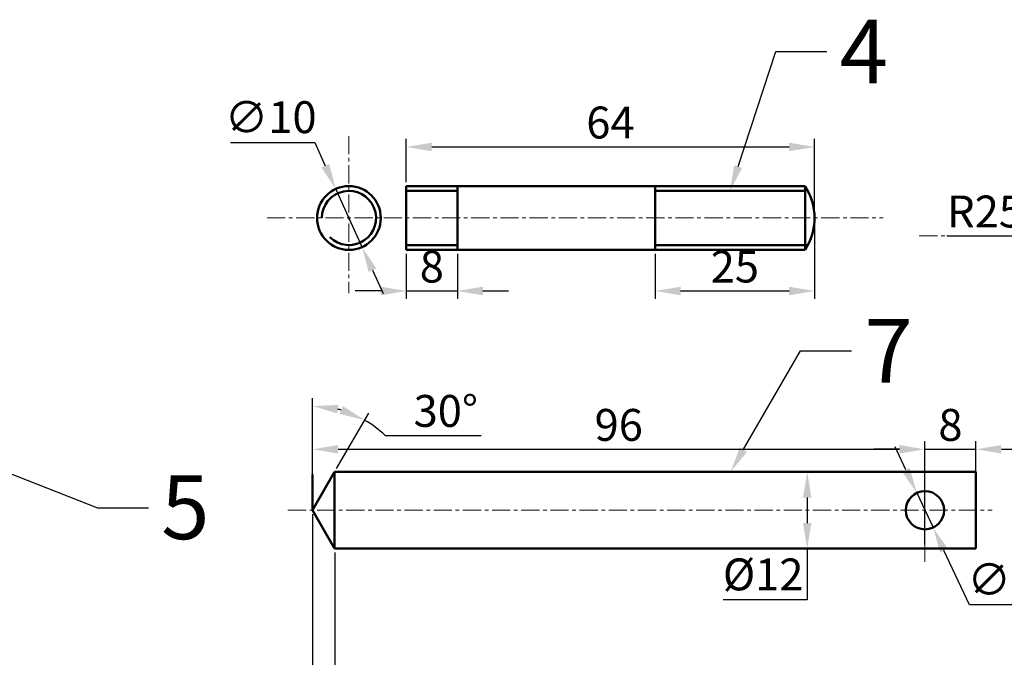
# Model space of a CAD drawing. Units: millimetres. Extents: x 24 to 508, y -182 to 223.
# Tile 4 of 6: x 207 to 361, y -25 to 75. Entities that reach past the tile are written whole.
import ezdxf
from ezdxf import colors
from ezdxf.entities.mleader import LeaderData, LeaderLine
from ezdxf.math import Vec2, Vec3

# ---------------------------------------------------------------- set-up
doc = ezdxf.new("R2010")
doc.units = ezdxf.units.MM
doc.header["$LTSCALE"] = 0.3
doc.linetypes.add('CENTER', pattern=[50.8, 31.75, -6.35, 6.35, -6.35])
for name, color, linetype, lineweight in [('M-CNTR', 1, 'CENTER', 18), ('M-DIMS', 2, 'Continuous', 25), ('M-OUTL', 7, 'Continuous', 50)]:
    doc.layers.add(name, color=color, linetype=linetype, lineweight=lineweight)
doc.styles.get("Standard").update_dxf_attribs({"font": 'arial.ttf'})
doc.dimstyles.new('ISO-25', dxfattribs={"dimtxt": 5, "dimasz": 4, "dimexe": 1.25, "dimexo": 0.625, "dimtad": 1, "dimtoh": 1, "dimdec": 0, "dimtxsty": 'Standard', "dimcen": 2.5, "dimadec": 0, "dimazin": 0, "dimtfac": 1, "dimtdec": 0, "dimtmove": 0, "dimatfit": 3, "dimfxl": 1, "dimarcsym": 0})

# ---------------------------------------------------------------- blocks, each defined once
blk = doc.blocks.new('*D30')
at = {"layer": 'Defpoints', "color": 0, "ltscale": 0.3, "transparency": 16777216}
for p in [(267.18, 38.45), (275.18, 38.45), (275.18, 32)]:
    blk.add_point(p, dxfattribs=at)
at = {"layer": 'M-DIMS', "color": 0, "lineweight": -2, "ltscale": 0.3, "transparency": 16777216}
for p, q in [((267.18, 37.82), (267.18, 30.75)), ((275.18, 37.82), (275.18, 30.75)), ((263.18, 32), (259.18, 32)), ((267.18, 32), (275.18, 32)), ((279.18, 32), (283.18, 32))]:
    blk.add_line(p, q, dxfattribs=at)
at = {"layer": 'M-DIMS', "color": 0, "ltscale": 0.3, "transparency": 16777216}
for points in [[(263.18, 32.67), (263.18, 31.33), (267.18, 32)], [(279.18, 32.67), (279.18, 31.33), (275.18, 32)]]:
    blk.add_solid(points, dxfattribs=at)
at = {"layer": 'M-DIMS', "color": 0, "ltscale": 0.3, "transparency": 16777216, "insert": (271.18, 35.18), "char_height": 5, "attachment_point": 5}
blk.add_mtext('8', dxfattribs=at)
blk = doc.blocks.new('*D31')
at = {"layer": 'Defpoints', "color": 0, "ltscale": 0.3, "transparency": 16777216}
for p in [(331.18, 43.45), (306.18, 38.45), (331.18, 32)]:
    blk.add_point(p, dxfattribs=at)
at = {"layer": 'M-DIMS', "color": 0, "lineweight": -2, "ltscale": 0.3, "transparency": 16777216}
for p, q in [((331.18, 42.82), (331.18, 30.75)), ((306.18, 37.82), (306.18, 30.75)), ((310.18, 32), (327.18, 32))]:
    blk.add_line(p, q, dxfattribs=at)
at = {"layer": 'M-DIMS', "color": 0, "ltscale": 0.3, "transparency": 16777216}
for points in [[(310.18, 32.67), (310.18, 31.33), (306.18, 32)], [(327.18, 32.67), (327.18, 31.33), (331.18, 32)]]:
    blk.add_solid(points, dxfattribs=at)
at = {"layer": 'M-DIMS', "color": 0, "ltscale": 0.3, "transparency": 16777216, "insert": (318.68, 35.18), "char_height": 5, "attachment_point": 5}
blk.add_mtext('25', dxfattribs=at)
blk = doc.blocks.new('*D32')
at = {"layer": 'Defpoints', "color": 0, "ltscale": 0.3, "transparency": 16777216}
for p in [(331.18, 54.59), (267.18, 48.45), (331.18, 43.45)]:
    blk.add_point(p, dxfattribs=at)
at = {"layer": 'M-DIMS', "color": 0, "lineweight": -2, "ltscale": 0.3, "transparency": 16777216}
for p, q in [((267.18, 49.07), (267.18, 55.84)), ((331.18, 44.07), (331.18, 55.84)), ((271.18, 54.59), (327.18, 54.59))]:
    blk.add_line(p, q, dxfattribs=at)
at = {"layer": 'M-DIMS', "color": 0, "ltscale": 0.3, "transparency": 16777216}
for points in [[(271.18, 55.26), (271.18, 53.92), (267.18, 54.59)], [(327.18, 55.26), (327.18, 53.92), (331.18, 54.59)]]:
    blk.add_solid(points, dxfattribs=at)
at = {"layer": 'M-DIMS', "color": 0, "ltscale": 0.3, "transparency": 16777216, "insert": (299.18, 57.77), "char_height": 5, "attachment_point": 5}
blk.add_mtext('64', dxfattribs=at)
blk = doc.blocks.new('*D33')
at = {"layer": 'Defpoints', "color": 0, "ltscale": 0.3, "transparency": 16777216}
for p in [(256.12, 48), (260.24, 38.89)]:
    blk.add_point(p, dxfattribs=at)
at = {"layer": 'M-DIMS', "color": 0, "lineweight": -2, "ltscale": 0.3, "transparency": 16777216}
for p, q in [((239.62, 55.3), (252.83, 55.3)), ((252.83, 55.3), (254.48, 51.65)), ((260.24, 38.89), (256.12, 48)), ((261.88, 35.24), (263.53, 31.6))]:
    blk.add_line(p, q, dxfattribs=at)
at = {"layer": 'M-DIMS', "color": 0, "ltscale": 0.3, "transparency": 16777216}
for points in [[(255.09, 51.92), (253.87, 51.38), (256.12, 48)], [(262.49, 35.52), (261.28, 34.97), (260.24, 38.89)]]:
    blk.add_solid(points, dxfattribs=at)
at = {"layer": 'M-DIMS', "color": 0, "ltscale": 0.3, "transparency": 16777216, "insert": (245.92, 58.61), "char_height": 5, "attachment_point": 5}
blk.add_mtext('∅10', dxfattribs=at)
blk = doc.blocks.new('*D34')
at = {"layer": 'Defpoints', "color": 0, "ltscale": 0.3, "transparency": 16777216}
for p in [(255.32, 13.71), (252.48, 3.24), (255.95, 3.61), (252.48, -2.39), (252.48, -2.39)]:
    blk.add_point(p, dxfattribs=at)
at = {"layer": 'M-DIMS', "color": 0, "lineweight": -2, "ltscale": 0.3, "transparency": 16777216}
for p, q in [((252.48, 3.87), (252.48, 15.2)), ((256.26, 4.16), (261.28, 12.85)), ((263.85, 9.36), (278.9, 9.36))]:
    blk.add_line(p, q, dxfattribs=at)
for start, end in [(74.0616, 75.9384), (45.9384, 60)]:
    blk.add_arc((252.48, -2.39), 16.34, start, end, dxfattribs=at)
at = {"layer": 'M-DIMS', "color": 0, "ltscale": 0.3, "transparency": 16777216}
for points in [[(256.37, 12.8), (256.53, 14.13), (252.48, 13.95)], [(257.23, 13.94), (256.71, 12.71), (260.65, 11.77)]]:
    blk.add_solid(points, dxfattribs=at)
at = {"layer": 'M-DIMS', "color": 0, "ltscale": 0.3, "transparency": 16777216, "insert": (273.37, 12.54), "char_height": 5, "attachment_point": 5}
blk.add_mtext('30°', dxfattribs=at)
blk = doc.blocks.new('*D35')
at = {"layer": 'Defpoints', "color": 0, "ltscale": 0.3, "transparency": 16777216}
for p in [(348.48, 7.17), (252.48, -2.39), (348.48, -2.39)]:
    blk.add_point(p, dxfattribs=at)
at = {"layer": 'M-DIMS', "color": 0, "lineweight": -2, "ltscale": 0.3, "transparency": 16777216}
for p, q in [((252.48, -1.76), (252.48, 8.42)), ((348.48, -1.77), (348.48, 8.42)), ((256.48, 7.17), (344.48, 7.17))]:
    blk.add_line(p, q, dxfattribs=at)
at = {"layer": 'M-DIMS', "color": 0, "ltscale": 0.3, "transparency": 16777216}
for points in [[(256.48, 7.84), (256.48, 6.51), (252.48, 7.17)], [(344.48, 7.84), (344.48, 6.51), (348.48, 7.17)]]:
    blk.add_solid(points, dxfattribs=at)
at = {"layer": 'M-DIMS', "color": 0, "ltscale": 0.3, "transparency": 16777216, "insert": (300.48, 10.35), "char_height": 5, "attachment_point": 5}
blk.add_mtext('96', dxfattribs=at)
blk = doc.blocks.new('*D36')
at = {"layer": 'Defpoints', "color": 0, "ltscale": 0.3, "transparency": 16777216}
for p in [(356.48, 7.17), (348.48, -8.39), (356.48, -8.39)]:
    blk.add_point(p, dxfattribs=at)
at = {"layer": 'M-DIMS', "color": 0, "lineweight": -2, "ltscale": 0.3, "transparency": 16777216}
for p, q in [((348.48, -7.76), (348.48, 8.42)), ((356.48, -7.76), (356.48, 8.42)), ((344.48, 7.17), (340.48, 7.17)), ((348.48, 7.17), (356.48, 7.17)), ((360.48, 7.17), (364.48, 7.17))]:
    blk.add_line(p, q, dxfattribs=at)
at = {"layer": 'M-DIMS', "color": 0, "ltscale": 0.3, "transparency": 16777216}
for points in [[(344.48, 7.84), (344.48, 6.51), (348.48, 7.17)], [(360.48, 7.84), (360.48, 6.51), (356.48, 7.17)]]:
    blk.add_solid(points, dxfattribs=at)
at = {"layer": 'M-DIMS', "color": 0, "ltscale": 0.3, "transparency": 16777216, "insert": (352.48, 10.35), "char_height": 5, "attachment_point": 5}
blk.add_mtext('8', dxfattribs=at)
blk = doc.blocks.new('*D37')
at = {"layer": 'Defpoints', "color": 0, "ltscale": 0.3, "transparency": 16777216}
for p in [(330.03, 3.61), (332.02, 3.61), (332.02, -8.39)]:
    blk.add_point(p, dxfattribs=at)
at = {"layer": 'M-DIMS', "color": 0, "lineweight": -2, "ltscale": 0.3, "transparency": 16777216}
for p, q in [((331.39, 3.61), (328.78, 3.61)), ((330.03, -0.39), (330.03, -4.39)), ((331.39, -8.39), (328.78, -8.39)), ((330.03, -8.39), (330.03, -16.42)), ((330.03, -16.42), (316.85, -16.42))]:
    blk.add_line(p, q, dxfattribs=at)
at = {"layer": 'M-DIMS', "color": 0, "ltscale": 0.3, "transparency": 16777216}
for points in [[(329.36, -0.39), (330.69, -0.39), (330.03, 3.61)], [(329.36, -4.39), (330.69, -4.39), (330.03, -8.39)]]:
    blk.add_solid(points, dxfattribs=at)
at = {"layer": 'M-DIMS', "color": 0, "ltscale": 0.3, "transparency": 16777216, "insert": (323.12, -13.1), "char_height": 5, "attachment_point": 5}
blk.add_mtext('%%C12', dxfattribs=at)
blk = doc.blocks.new('*D38')
at = {"layer": 'Defpoints', "color": 0, "ltscale": 0.3, "transparency": 16777216}
for p in [(347.2, 0.33), (349.76, -5.1)]:
    blk.add_point(p, dxfattribs=at)
at = {"layer": 'M-DIMS', "color": 0, "lineweight": -2, "ltscale": 0.3, "transparency": 16777216}
for p, q in [((345.5, 3.95), (343.8, 7.57)), ((347.2, 0.33), (349.76, -5.1)), ((355.46, -17.21), (351.47, -8.72)), ((364.8, -17.21), (355.46, -17.21))]:
    blk.add_line(p, q, dxfattribs=at)
at = {"layer": 'M-DIMS', "color": 0, "ltscale": 0.3, "transparency": 16777216}
for points in [[(346.1, 4.23), (344.9, 3.66), (347.2, 0.33)], [(352.07, -8.43), (350.86, -9), (349.76, -5.1)]]:
    blk.add_solid(points, dxfattribs=at)
at = {"layer": 'M-DIMS', "color": 0, "ltscale": 0.3, "transparency": 16777216, "insert": (360.45, -13.89), "char_height": 5, "attachment_point": 5}
blk.add_mtext('∅6', dxfattribs=at)
blk = doc.blocks.new('*D74')
at = {"layer": 'Defpoints', "color": 0, "ltscale": 0.3, "transparency": 16777216}
for p in [(252.48, -2.39), (255.95, -8.39), (255.95, -174.63)]:
    blk.add_point(p, dxfattribs=at)
at = {"layer": 'M-DIMS', "color": 0, "lineweight": -2, "ltscale": 0.3, "transparency": 16777216}
for p, q in [((252.48, -3.01), (252.48, -175.88)), ((255.95, -9.01), (255.95, -175.88)), ((248.48, -174.63), (244.48, -174.63)), ((252.48, -174.63), (255.95, -174.63)), ((259.95, -174.63), (282.05, -174.63))]:
    blk.add_line(p, q, dxfattribs=at)
at = {"layer": 'M-DIMS', "color": 0, "ltscale": 0.3, "transparency": 16777216}
for points in [[(248.48, -173.96), (248.48, -175.3), (252.48, -174.63)], [(259.95, -173.96), (259.95, -175.3), (255.95, -174.63)]]:
    blk.add_solid(points, dxfattribs=at)
at = {"layer": 'M-DIMS', "color": 0, "ltscale": 0.3, "transparency": 16777216, "insert": (273, -171.45), "char_height": 5, "attachment_point": 5}
blk.add_mtext('3.464', dxfattribs=at)
blk = doc.blocks.new('*D83')
at = {"layer": 'Defpoints', "color": 0, "ltscale": 0.3, "transparency": 16777216}
for p in [(379.52, 40.64), (404.52, 40.64)]:
    blk.add_point(p, dxfattribs=at)
at = {"layer": 'M-DIMS', "color": 0, "lineweight": -2, "ltscale": 0.3, "transparency": 16777216}
for p, q in [((351.91, 40.64), (364.52, 40.64)), ((364.52, 40.64), (375.52, 40.64)), ((404.52, 40.64), (379.52, 40.64))]:
    blk.add_line(p, q, dxfattribs=at)
at = {"layer": 'M-DIMS', "color": 0, "ltscale": 0.3, "transparency": 16777216}
blk.add_solid([(375.52, 41.31), (375.52, 39.98), (379.52, 40.64)], dxfattribs=at)
at = {"layer": 'M-DIMS', "color": 0, "ltscale": 0.3, "transparency": 16777216, "insert": (357.9, 43.82), "char_height": 5, "attachment_point": 5}
blk.add_mtext('R25', dxfattribs=at)

msp = doc.modelspace()

# ---------------------------------------------------------------- linework, layer by layer
at = {"layer": 'M-CNTR', "ltscale": 0.3}
for p, q in [((258.1817, 56.2933), (258.1817, 31.6591)), ((245.3504, 43.4473), (341.9324, 43.4473)), ((428.1856, 40.6427), (347.5151, 40.6427)), ((348.4824, 6.0945), (348.4824, -10.8826)), ((248.6176, -2.3853), (359.0359, -2.3853))]:
    msp.add_line(p, q, dxfattribs=at)
at = {"layer": 'M-OUTL', "ltscale": 0.3}
for p, q in [((267.1831, 48.4473), (267.1831, 38.4473)), ((329.6831, 48.4473), (267.1831, 48.4473)), ((275.1831, 48.4473), (275.1831, 38.4473)), ((306.1831, 38.4473), (306.1831, 48.4473)), ((329.6831, 38.4473), (329.6831, 48.4473)), ((275.1831, 47.6973), (267.1831, 47.6973)), ((329.6831, 47.6973), (306.1831, 47.6973)), ((267.1831, 39.1973), (275.1831, 39.1973)), ((306.1831, 39.1973), (330.1275, 39.1973)), ((267.1831, 38.4473), (329.6831, 38.4473)), ((252.4824, -2.3853), (255.9466, 3.6147)), ((252.4824, -2.3853), (252.4824, 3.2442)), ((255.9466, 3.6147), (255.9466, -8.3853)), ((356.4824, 3.6147), (255.9466, 3.6147)), ((356.4824, -8.3853), (356.4824, 3.6147)), ((252.4824, -2.3853), (255.9466, -8.3853)), ((255.9466, -8.3853), (356.4824, -8.3853))]:
    msp.add_line(p, q, dxfattribs=at)
for centre, radius in [((258.1817, 43.4473), 5), ((348.4824, -2.3853), 3)]:
    msp.add_circle(centre, radius, dxfattribs=at)
for centre, radius, start, end in [((322.0997, 43.4473), 9.0833, 326.601512, 33.398488), ((258.1817, 43.4473), 4.25, 225, 180)]:
    msp.add_arc(centre, radius, start, end, dxfattribs=at)

# ---------------------------------------------------------------- dimensions: what is measured, and where the dimension line sits
at = {"layer": 'M-DIMS', "ltscale": 0.3}
for p1, p2, picture, middle in [((260.2387, 38.8899), (256.1248, 48.0046), '*D33', (245.9161, 58.614)), ((347.2042, 0.3287), (349.7607, -5.0994), '*D38', (360.446, -13.8913))]:
    dim = msp.add_diameter_dim_2p(p1=p1, p2=p2, dimstyle='ISO-25', override={"dimclrd": 0, "dimclre": 0, "dimclrt": 0}, dxfattribs=at)
    dim.commit()
    dim.dimension.update_dxf_attribs({"geometry": picture, "text_midpoint": middle})
for base, p1, p2, override, picture, middle in [((331.1831, 54.5885), (267.1831, 48.4473), (331.1831, 43.4473), {"dimclrd": 0, "dimclre": 0, "dimclrt": 0}, '*D32', (299.1831, 57.7664)), ((331.1831, 32), (306.1831, 38.4473), (331.1831, 43.4473), {"dimclrd": 0, "dimclre": 0, "dimclrt": 0}, '*D31', (318.6831, 35.1779)), ((275.1831, 32), (267.1831, 38.4473), (275.1831, 38.4473), {"dimclrd": 0, "dimclre": 0, "dimclrt": 0}, '*D30', (271.1831, 35.1779)), ((348.4824, 7.1732), (252.4824, -2.3853), (348.4824, -2.394), {"dimclrd": 0, "dimclre": 0, "dimclrt": 0}, '*D35', (300.4824, 10.3511)), ((356.4824, 7.1732), (348.4824, -8.3853), (356.4824, -8.3853), {"dimclrd": 0, "dimclre": 0, "dimclrt": 0}, '*D36', (352.4824, 10.3511)), ((255.9466, -174.6307), (252.4824, -2.3853), (255.9466, -8.3853), {"dimdec": 3, "dimlfac": 1, "dimrnd": 0, "dimzin": 0, "dimdsep": 46, "dimlunit": 2}, '*D74', (272.9958, -171.4511))]:
    dim = msp.add_linear_dim(base=base, p1=p1, p2=p2, dimstyle='ISO-25', override=override, dxfattribs=at)
    dim.commit()
    dim.dimension.update_dxf_attribs({"geometry": picture, "text_midpoint": middle})
dim = msp.add_radius_dim(center=(404.5166, 40.6427), mpoint=(379.5166, 40.643), dimstyle='ISO-25', override={"dimdec": 0, "dimlfac": 1, "dimrnd": 0, "dimzin": 0, "dimdsep": 46, "dimlunit": 2}, dxfattribs=at)
dim.commit()
dim.dimension.update_dxf_attribs({"geometry": '*D83', "text_midpoint": (364.5166, 40.6432), "dimtype": 164})
dim = msp.add_angular_dim_2l(base=(255.3198, 13.7059), line1=((252.4824, -2.3853), (255.9466, 3.6147)), line2=((252.4824, -2.3853), (252.4824, 3.2442)), dimstyle='ISO-25', override={"dimclrd": 0, "dimclre": 0, "dimclrt": 0}, dxfattribs=at)
dim.commit()
dim.dimension.update_dxf_attribs({"geometry": '*D34', "text_midpoint": (273.3732, 12.5357)})
dim = msp.add_linear_dim(base=(330.0252, 3.6147), p1=(332.0151, -8.3853), p2=(332.0151, 3.6147), angle=90, text='%%C<>', dimstyle='ISO-25', override={"dimclrd": 0, "dimclre": 0, "dimclrt": 0}, dxfattribs=at)
dim.commit()
dim.dimension.update_dxf_attribs({"geometry": '*D37', "text_midpoint": (323.1247, -16.4185), "dimtype": 160})

# ---------------------------------------------------------------- leaders
ml = msp.add_multileader_mtext('Standard', dxfattribs=at)
ml.set_content('4', color=256)
ml.set_leader_properties()
ml.build(insert=Vec2(0, 0))
ctx = ml.context
ctx.base_point, ctx.char_height, ctx.plane_origin = Vec3(333.123, 69.5474), 10, Vec3(317.9331, 47.6973)
notes = []
notes.append((ctx, [(0, (1, 1, 0), (325.123, 69.5474), (1, 0), 8, [(0, [(317.9331, 47.6973)], 0, [])])]))
ctx.mtext.insert, ctx.mtext.flow_direction = Vec3(335.123, 74.5474), 5
ml = msp.add_multileader_mtext('Standard', dxfattribs=at)
ml.set_content('7', color=256)
ml.set_leader_properties()
ml.build(insert=Vec2(0, 0))
ctx = ml.context
ctx.base_point, ctx.char_height, ctx.plane_origin = Vec3(336.9852, 22.6257), 10, Vec3(318.0091, 3.6147)
notes.append((ctx, [(0, (1, 1, 0), (328.9852, 22.6257), (1, 0), 8, [(0, [(318.0091, 3.6147)], 0, [])])]))
ctx.mtext.insert, ctx.mtext.flow_direction = Vec3(338.9852, 27.6257), 5
ml = msp.add_multileader_mtext('Standard', dxfattribs=at)
ml.set_content('5', color=256)
ml.set_leader_properties()
ml.build(insert=Vec2(0, 0))
ctx = ml.context
ctx.base_point, ctx.char_height, ctx.plane_origin = Vec3(226.7556, -2.0023), 10, Vec3(190.3582, 7.9426)
notes.append((ctx, [(0, (1, 1, 0), (218.7556, -2.0023), (1, 0), 8, [(0, [(188.3582, 9.9426)], 0, [])])]))
ctx.mtext.insert, ctx.mtext.flow_direction = Vec3(228.7556, 3.083), 5
for ctx, leaders in notes:
    for number, flags, end, landing, length, lines in leaders:
        leader = LeaderData()
        leader.index, (leader.has_last_leader_line, leader.has_dogleg_vector, leader.attachment_direction) = number, flags
        leader.last_leader_point, leader.dogleg_vector, leader.dogleg_length = Vec3(end), Vec3(landing), length
        for number, points, colour, breaks in lines:
            line = LeaderLine()
            line.index, line.vertices, line.color, line.breaks = number, Vec3.list(points), colors.encode_raw_color(colour), breaks
            leader.lines.append(line)
        ctx.leaders.append(leader)

doc.saveas('drawing.dxf')
